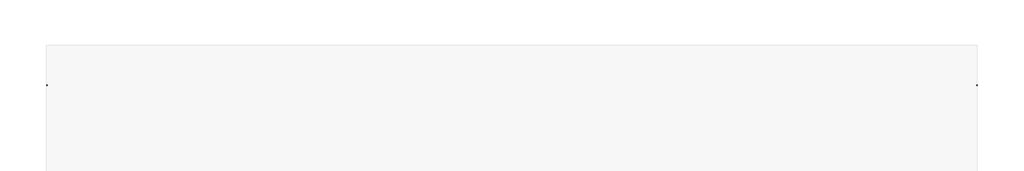
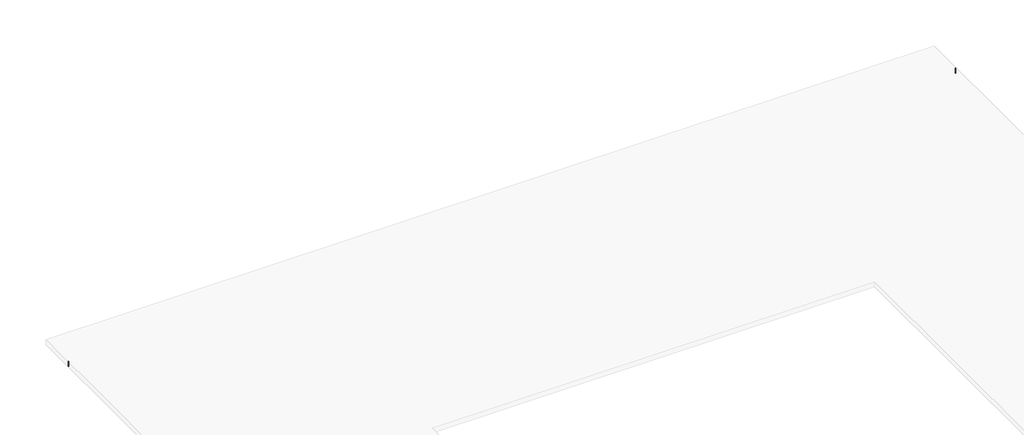
# One storey, part 2 of 2: 1 reinforcing bar.
"""IFC4 building model written with IfcOpenShell, lengths in millimetres."""

from ifc_helpers import new_model, si_unit, origin, place, context, project, spatial, polyline, segment, composite_curve, source, transform, mapped, element, save
from ifc_brep_helpers import swept_disk

model = new_model("IFC4")

# Units and contexts
model_context = context("Model", 3, world=origin())
ifc_project = project(units=[si_unit("LENGTHUNIT", "METRE", prefix="MILLI")], contexts=[model_context])

# Site, building, storey
site = spatial("IfcSite", under=ifc_project)
building = spatial("IfcBuilding", under=site)
storey = spatial("IfcBuildingStorey", under=building, Elevation=-2000.0)

# Reinforcing bar
placement = place(None, origin())
reinforcing_bar_shape = source(origin(), model_context, "Body", "SolidModel", [
    swept_disk(composite_curve([segment(polyline([(22049.1673137, 14533.7790238, -2280.0), (22049.1673137, 14533.7790238, -2020.0)]), True, "CONTINUOUS")], self_intersect=False), 10.0),
])
element("IfcReinforcingBar", 1, at=placement, inside=storey, context=model_context, shape_type="MappedRepresentation", body=[
    mapped(reinforcing_bar_shape, transform((0.0, 0.0, 0.0), x_axis=(1.0, 0.0, 0.0), y_axis=(0.0, 1.0, 0.0), z_axis=(0.0, 0.0, 1.0))),
    mapped(reinforcing_bar_shape, transform((-47920.0, 0.0, 0.0), x_axis=(1.0, 0.0, 0.0), y_axis=(0.0, 1.0, 0.0), z_axis=(0.0, 0.0, 1.0))),
])

save(model, "model.ifc")

# Revit data of these elements
# Element 1 (IfcReinforcingBar)
#   Phase Created = New Construction
